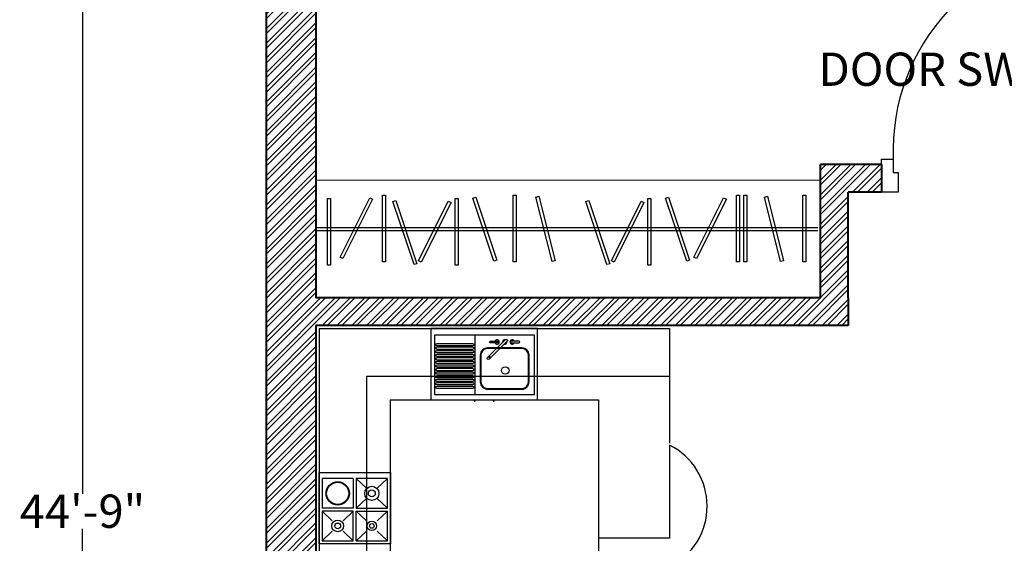
# Model space of a CAD drawing. Units: inches. Extents: x 528 to 2520, y -151 to 1354.
# Tile 2 of 41: x 542 to 720, y 1043 to 1137. Entities that reach past the tile are written whole.
import ezdxf

# ---------------------------------------------------------------- set-up
doc = ezdxf.new("R2010")
doc.units = ezdxf.units.IN
doc.header["$MEASUREMENT"] = 0
for name, color, linetype, lineweight in [('A-ANNO-DIMS', 2, 'Continuous', 18), ('A-Door', 150, 'Continuous', 25), ('A-FLOR-CASE', 11, 'Continuous', 20), ('A-WALL-PATT', 6, 'Continuous', 13), ('walls', 7, 'Continuous', 40)]:
    doc.layers.add(name, color=color, linetype=linetype, lineweight=lineweight)
for name, color, linetype in [('ESYA', 11, 'Continuous'), ('HID', 11, 'Continuous'), ('NT', 1, 'Continuous'), ('TEFRIS', 11, 'Continuous')]:
    doc.layers.add(name, color=color, linetype=linetype)
doc.styles.get("Standard").update_dxf_attribs({"font": 'arial.ttf'})
doc.dimstyles.get("Standard").update_dxf_attribs({"dimtxt": 6, "dimasz": 2, "dimexe": 0.18, "dimexo": 0.0625, "dimgap": 0.09, "dimtad": 0, "dimtih": 1, "dimtoh": 1, "dimdec": 1, "dimzin": 0, "dimdsep": 46, "dimlunit": 3, "dimtxsty": 'Standard', "dimblk": 'ARCHTICK', "dimcen": 0.09, "dimadec": 0, "dimazin": 0, "dimtfac": 1, "dimtdec": 1, "dimtofl": 0, "dimtmove": 0, "dimatfit": 3, "dimfxl": 1, "dimtolj": 1, "dimtzin": 0, "dimarcsym": 0})

# ---------------------------------------------------------------- blocks, each defined once
blk = doc.blocks.new('A$C7DB75F4D')
at = {"layer": 'A-Door'}
for points in [[(625, 740), (625, 660), (665, 660), (665, 740)], [(625, 180), (625, 660), (665, 660), (665, 180)], [(625, 100), (625, 180), (665, 180), (665, 100)], [(35, 100), (35, 60), (50, 60), (50, 50), (50, 0), (0, 0), (0, 100)], [(665, 100), (700, 100), (700, 0), (650, 0), (650, 50), (650, 60), (665, 60)]]:
    blk.add_lwpolyline(points, close=True, dxfattribs=at)
at = {"layer": 'NT'}
blk.add_arc((650, 125), 615.5, 92.3278, 182.3278, dxfattribs=at)
blk = doc.blocks.new('A$C41BE763B')
at = {"layer": 'HID'}
for p, q in [((3.395, 0.2532), (0, 0.2532)), ((3.395, 0.2332), (0, 0.2332))]:
    blk.add_line(p, q, dxfattribs=at)
for points in [[(0.4716, 0.4734), (0.4716, 0.0234), (0.4508, 0.0234), (0.4508, 0.4734)], [(1.3547, 0.4734), (1.3547, 0.0234), (1.3339, 0.0234), (1.3339, 0.4734)], [(2.8639, 0.4734), (2.8639, 0.0234), (2.8432, 0.0234), (2.8432, 0.4734)], [(2.9139, 0.4734), (2.9139, 0.0234), (2.8932, 0.0234), (2.8932, 0.4734)], [(3.3139, 0.4734), (3.3139, 0.0234), (3.2932, 0.0234), (3.2932, 0.4734)], [(0.0983, 0.45), (0.0983, 0), (0.0775, 0), (0.0775, 0.45)], [(0.3834, 0.447), (0.1822, 0.0445), (0.1636, 0.0538), (0.3648, 0.4563)], [(0.5408, 0.4372), (0.6831, 0.0103), (0.6634, 0.0037), (0.5211, 0.4306)], [(0.914, 0.4236), (0.7128, 0.0211), (0.6942, 0.0304), (0.8954, 0.4329)], [(0.9617, 0.45), (0.9617, 0), (0.941, 0), (0.941, 0.45)], [(1.0809, 0.4606), (1.2232, 0.0337), (1.2035, 0.0271), (1.0612, 0.454)], [(1.5084, 0.466), (1.6175, 0.0294), (1.5974, 0.0244), (1.4882, 0.4609)], [(1.8448, 0.4372), (1.9871, 0.0103), (1.9674, 0.0037), (1.8251, 0.4306)], [(2.218, 0.4236), (2.0167, 0.0211), (1.9981, 0.0304), (2.1994, 0.4329)], [(2.2657, 0.45), (2.2657, 0), (2.2449, 0), (2.2449, 0.45)], [(2.3849, 0.4606), (2.5272, 0.0337), (2.5075, 0.0271), (2.3652, 0.454)], [(2.7757, 0.447), (2.5745, 0.0445), (2.5559, 0.0538), (2.7572, 0.4563)], [(3.0533, 0.466), (3.1624, 0.0294), (3.1423, 0.0244), (3.0332, 0.4609)]]:
    blk.add_lwpolyline(points, close=True, dxfattribs=at)
blk = doc.blocks.new('AR365L')
blk.add_line((0, 0.0995), (0.61, 0.0995))
blk.add_lwpolyline([(0, 0), (0, 0.68), (0.61, 0.68), (0.61, 0)], close=True)
blk = doc.blocks.new('FIRIN1')
at = {"layer": 'ESYA'}
for p, q in [((0.2875, -0.05), (0.2875, -0.3006)), ((0.3983, -0.1319), (0.3125, -0.05)), ((0.575, -0.05), (0.4892, -0.1319)), ((0.3983, -0.2187), (0.3125, -0.3006)), ((0.575, -0.3006), (0.4892, -0.2187)), ((0.2875, -0.3006), (0.025, -0.3006)), ((0.025, -0.3244), (0.1108, -0.4063)), ((0.2017, -0.4063), (0.2875, -0.3244)), ((0.3983, -0.4063), (0.3125, -0.3244)), ((0.575, -0.3244), (0.4892, -0.4063)), ((0.025, -0.575), (0.1108, -0.4931)), ((0.2017, -0.4931), (0.2875, -0.575)), ((0.3983, -0.4931), (0.3125, -0.575)), ((0.575, -0.575), (0.4892, -0.4931))]:
    blk.add_line(p, q, dxfattribs=at)
blk.add_lwpolyline([(0, 0), (0.6, 0), (0.6, -0.6), (0, -0.6)], close=True, dxfattribs=at)
for points in [[(0.2875, -0.05), (0.025, -0.05), (0.025, -0.3006)], [(0.3125, -0.05), (0.3125, -0.3006), (0.575, -0.3006)], [(0.575, -0.3006), (0.575, -0.05), (0.3125, -0.05)], [(0.2875, -0.575), (0.2875, -0.3244), (0.025, -0.3244)], [(0.025, -0.3244), (0.025, -0.575)], [(0.3125, -0.575), (0.3125, -0.3244), (0.575, -0.3244)], [(0.3125, -0.575), (0.575, -0.575), (0.575, -0.3244)], [(0.025, -0.575), (0.2875, -0.575)]]:
    blk.add_lwpolyline(points, dxfattribs=at)
for centre, radius in [((0.1562, -0.1753), 0.0986), ((0.1562, -0.1753), 0.0936), ((0.4438, -0.1753), 0.0597), ((0.4438, -0.1753), 0.0294), ((0.1562, -0.4497), 0.0492), ((0.4438, -0.4497), 0.0398), ((0.1562, -0.4497), 0.0242), ((0.4438, -0.4497), 0.0196)]:
    blk.add_circle(centre, radius, dxfattribs=at)
blk = doc.blocks.new('ncvn')
for p, q in [((77868.38, -4466.7), (77868.38, -4520.7)), ((77949.38, -4466.7), (77868.38, -4466.7)), ((77949.38, -4520.7), (77949.38, -4466.7))]:
    blk.add_line(p, q)
at = {"layer": 'TEFRIS'}
for p, q in [((77783.66, -4466.69), (77783.66, -4763.38)), ((77783.66, -4466.69), (78049.52, -4466.69)), ((77901.95, -4516.62), (77901.95, -4471.62)), ((78049.52, -4466.69), (78049.52, -4553.55)), ((77819.66, -4502.83), (77819.66, -4759.23)), ((77819.66, -4502.83), (78049.52, -4502.83)), ((77837.66, -4520.83), (77837.66, -4704.71)), ((77837.66, -4520.83), (77995.52, -4520.83)), ((77868.38, -4520.7), (77949.38, -4520.7)), ((77995.52, -4520.83), (77995.52, -4642.99)), ((78049.52, -4554.99), (78049.52, -4625.66)), ((78049.52, -4625.66), (77995.83, -4625.66)), ((77783.66, -4704.71), (77837.66, -4704.71))]:
    blk.add_line(p, q, dxfattribs=at)
for points in [[(77868.38, -4466.7), (77868.38, -4520.7), (77949.38, -4520.7), (77949.38, -4466.7)], [(77871.35, -4471.62), (77871.35, -4516.62), (77946.95, -4516.62), (77946.95, -4471.62)]]:
    blk.add_lwpolyline(points, close=True, dxfattribs=at)
for points in [[(77873.15, -4477.92), (77900.15, -4477.92, -1), (77900.15, -4479.72), (77873.15, -4479.72, -1), (77873.15, -4477.92)], [(77873.15, -4480.62), (77900.15, -4480.62, -1), (77900.15, -4482.42), (77873.15, -4482.42, -1), (77873.15, -4480.62)], [(77873.15, -4483.32), (77900.15, -4483.32, -1), (77900.15, -4485.12), (77873.15, -4485.12, -1), (77873.15, -4483.32)], [(77873.15, -4486.02), (77900.15, -4486.02, -1), (77900.15, -4487.82), (77873.15, -4487.82, -1), (77873.15, -4486.02)], [(77873.15, -4488.72), (77900.15, -4488.72, -1), (77900.15, -4490.52), (77873.15, -4490.52, -1), (77873.15, -4488.72)], [(77873.15, -4491.42), (77900.15, -4491.42, -1), (77900.15, -4493.22), (77873.15, -4493.22, -1), (77873.15, -4491.42)], [(77873.15, -4494.12), (77900.15, -4494.12, -1), (77900.15, -4495.92), (77873.15, -4495.92, -1), (77873.15, -4494.12)], [(77873.15, -4496.82), (77900.15, -4496.82, -1), (77900.15, -4498.62), (77873.15, -4498.62, -1), (77873.15, -4496.82)], [(77873.15, -4499.52), (77900.15, -4499.52, -1), (77900.15, -4501.32), (77873.15, -4501.32, -1), (77873.15, -4499.52)], [(77873.15, -4502.22), (77900.15, -4502.22, -1), (77900.15, -4504.02), (77873.15, -4504.02, -1), (77873.15, -4502.22)], [(77873.15, -4504.92), (77900.15, -4504.92, -1), (77900.15, -4506.72), (77873.15, -4506.72, -1), (77873.15, -4504.92)], [(77873.15, -4507.62), (77900.15, -4507.62, -1), (77900.15, -4509.42), (77873.15, -4509.42, -1), (77873.15, -4507.62)], [(77873.15, -4510.32), (77900.15, -4510.32, -1), (77900.15, -4512.12), (77873.15, -4512.12, -1), (77873.15, -4510.32)]]:
    blk.add_lwpolyline(points, format="xyb", dxfattribs=at)
for points in [[(77911.5, -4488.58), (77925.04, -4475.05, -1), (77926.25, -4476.26), (77912.72, -4489.8, -1)], [(77913.54, -4476.29), (77919.71, -4476.29, -0.563183), (77919.71, -4477.44), (77913.54, -4477.44, -1)], [(77935.33, -4476.29), (77929.17, -4476.29, 0.563183), (77929.17, -4477.44), (77935.33, -4477.44, 1)], [(77905.95, -4486.73), (77905.95, -4507.22, 0.414214), (77911.35, -4512.62), (77937.55, -4512.62, 0.414214), (77942.95, -4507.22), (77942.95, -4486.73, 0.414214), (77937.55, -4481.33), (77911.35, -4481.33, 0.414214)], [(77906.49, -4486.73), (77906.49, -4507.22, 0.414214), (77911.35, -4512.08), (77937.55, -4512.08, 0.414214), (77942.41, -4507.22), (77942.41, -4486.73, 0.414214), (77937.55, -4481.87), (77911.35, -4481.87, 0.414214)]]:
    blk.add_lwpolyline(points, format="xyb", close=True, dxfattribs=at)
for points in [[(77901.23, -4520.7), (77901.23, -4521.6), (77902.13, -4521.6), (77902.13, -4520.7)], [(77915.63, -4520.7), (77915.63, -4521.6), (77916.53, -4521.6), (77916.53, -4520.7)]]:
    blk.add_lwpolyline(points, dxfattribs=at)
for centre, radius in [((77913.01, -4488.3), 0.571), ((77924.89, -4498.48), 2.86)]:
    blk.add_circle(centre, radius, dxfattribs=at)
for centre, radius, start, end in [((77918.69, -4476.87), 1.71, 199.47122, 160.52878), ((77924.44, -4476.87), 1.71, 75, 195), ((77924.44, -4476.87), 1.71, 255, 15), ((77930.19, -4476.87), 1.71, 19.47122, 340.52878), ((78026.22, -4601.26), 51.8, 233.6588, 63.26709)]:
    blk.add_arc(centre, radius, start, end, dxfattribs=at)
at = {"layer": 'TEFRIS', "xscale": 90, "yscale": 90, "zscale": 90}
blk.add_blockref('FIRIN1', (77783.76, -4575.88), dxfattribs=at)
at = {"layer": 'TEFRIS', "xscale": 90, "yscale": 90, "zscale": 90, "rotation": 90}
blk.add_blockref('AR365L', (77848.22, -4760.91), dxfattribs=at)
blk = doc.blocks.new('_ArchTick')
at = {"color": 0, "linetype": 'ByBlock', "const_width": 0.15}
blk.add_lwpolyline([(-0.5, -0.5), (0.5, 0.5)], dxfattribs=at)
blk = doc.blocks.new('*D40')
at = {"layer": 'A-ANNO-DIMS', "color": 0, "lineweight": -2, "transparency": 16777216}
for p, q in [((744.63, 1150.5), (737.86, 1150.5)), ((738.04, 1150.5), (738.04, 1131.5)), ((738.04, 1106.1), (738.04, 1125.11)), ((744.63, 1106.1), (737.86, 1106.1))]:
    blk.add_line(p, q, dxfattribs=at)
at = {"layer": 'Defpoints', "color": 0, "transparency": 16777216}
for p in [(738.04, 1150.5), (744.7, 1150.5), (744.7, 1106.1)]:
    blk.add_point(p, dxfattribs=at)
at = {"layer": 'A-ANNO-DIMS', "color": 0, "lineweight": -2, "transparency": 16777216, "xscale": 2, "yscale": 2, "zscale": 2}
for p, rotation in [((738.04, 1150.5), 90), ((738.04, 1106.1), 270)]:
    blk.add_blockref('_ArchTick', p, dxfattribs=dict(at, rotation=rotation))
at = {"layer": 'A-ANNO-DIMS', "color": 0, "transparency": 16777216, "insert": (738.04, 1128.3), "char_height": 6, "attachment_point": 5}
blk.add_mtext('\\A1;DOOR SWING 3\'-8 1/2" TYP.', dxfattribs=at)
blk = doc.blocks.new('*D92')
at = {"layer": 'A-ANNO-DIMS', "color": 0, "lineweight": -2, "transparency": 16777216}
for p, q in [((586.63, 1317.1), (553.42, 1317.1)), ((553.6, 1317.1), (553.6, 1051.76)), ((553.6, 780.1), (553.6, 1045.45)), ((586.63, 780.1), (553.42, 780.1))]:
    blk.add_line(p, q, dxfattribs=at)
at = {"layer": 'Defpoints', "color": 0, "transparency": 16777216}
for p in [(553.6, 1317.1), (586.7, 1317.1), (586.7, 780.1)]:
    blk.add_point(p, dxfattribs=at)
at = {"layer": 'A-ANNO-DIMS', "color": 0, "lineweight": -2, "transparency": 16777216, "xscale": 2, "yscale": 2, "zscale": 2}
for p, rotation in [((553.6, 1317.1), 90), ((553.6, 780.1), 270)]:
    blk.add_blockref('_ArchTick', p, dxfattribs=dict(at, rotation=rotation))
at = {"layer": 'A-ANNO-DIMS', "color": 0, "transparency": 16777216, "insert": (553.6, 1048.6), "char_height": 6, "attachment_point": 5}
blk.add_mtext('\\A1;44\'-9"', dxfattribs=at)

msp = doc.modelspace()

# ---------------------------------------------------------------- hatches: boundary and pattern name
at = {"layer": 'A-WALL-PATT'}
h = msp.add_hatch(dxfattribs=at)
h.set_pattern_fill('ANSI32', color=256, scale=5)
h.paths.add_polyline_path([(595.7, 1163.86), (586.7, 1163.86), (586.7, 969.1), (598.24, 969.1), (603.24, 969.1), (603.24, 974.1), (595.7, 974.1), (595.7, 1082.1), (691.7, 1082.1), (691.7, 1087.1), (691.7, 1106.1), (697.7, 1106.1), (697.7, 1111.1), (686.7, 1111.1), (686.7, 1087.1), (595.7, 1087.1)])
h.paths.add_polyline_path([(688.7, 974.1), (651.24, 974.1), (651.24, 969.1), (688.7, 969.1)])
h.paths.add_polyline_path([(885.7, 1171.37), (876.7, 1171.37), (876.7, 1111.1), (786.7, 1111.1), (786.7, 1106.1), (876.7, 1106.1), (876.7, 974.1), (786.7, 974.1), (786.7, 969.1), (876.7, 969.1), (876.7, 825.1), (834.7, 825.1), (834.7, 816.1), (885.7, 816.1)])
h.paths.add_polyline_path([(885.7, 1317.1), (876.65, 1317.1), (876.65, 1308.1), (876.7, 1308.1), (876.7, 1248.1), (822.7, 1248.1), (822.7, 1243.1), (876.7, 1243.1), (876.7, 1219.37), (885.7, 1219.37)])
h.paths.add_polyline_path([(852.65, 1317.1), (787.7, 1317.1), (787.7, 1248.1), (784.26, 1248.1), (784.26, 1243.1), (792.7, 1243.1), (792.7, 1249.1), (792.7, 1308.1), (852.65, 1308.1)])
h.paths.add_polyline_path([(684.7, 1317.1), (619.7, 1317.1), (619.7, 1308.1), (679.7, 1308.1), (679.7, 1248.1), (679.7, 1243.1), (684.7, 1243.1), (684.7, 1248.25)])
h.paths.add_polyline_path([(595.7, 1308.1), (595.7, 1317.1), (586.7, 1317.1), (586.7, 1211.86), (595.7, 1211.86), (595.7, 1243.1), (649.7, 1243.1), (649.7, 1248.1), (595.7, 1248.1)])
h.paths.add_polyline_path([(744.7, 969.1), (744.7, 974.1), (724.7, 974.1), (724.7, 969.1), (739.7, 969.1), (739.7, 874.29), (744.7, 874.29)])
h.paths.add_polyline_path([(739.7, 969.1), (727.7, 969.1), (727.7, 965.12), (730.74, 965.12), (730.74, 961.68), (734.43, 961.68), (734.43, 957.24), (739.7, 957.24)], flags=17)
h.paths.add_polyline_path([(786.7, 825.1), (744.7, 825.1), (744.7, 832.29), (739.7, 832.29), (739.7, 816.1), (786.7, 816.1)])

# ---------------------------------------------------------------- linework, layer by layer
at = {"layer": 'A-FLOR-CASE'}
msp.add_line((595.7, 1108.27), (686.7, 1108.27), dxfattribs=at)
at = {"layer": 'walls'}
for p, q in [((586.7, 1317.1), (586.7, 789.1)), ((595.7, 1243.1), (595.7, 1087.1)), ((686.7, 1087.1), (686.7, 1111.1)), ((697.7, 1111.1), (686.7, 1111.1)), ((697.7, 1111.1), (697.7, 1106.1)), ((691.7, 1087.1), (691.7, 1106.1)), ((697.7, 1106.1), (691.7, 1106.1)), ((686.7, 1087.1), (595.7, 1087.1)), ((691.7, 1087.1), (691.7, 1082.1)), ((691.7, 1082.1), (595.7, 1082.1)), ((595.7, 1082.1), (595.7, 974.1))]:
    msp.add_line(p, q, dxfattribs=at)

# ---------------------------------------------------------------- block references
at = {"layer": 'A-Door', "xscale": 0.0600000000000059, "yscale": 0.0600000000000059, "zscale": 0.0600000000000059}
msp.add_blockref('A$C7DB75F4D', (697.7, 1106.1), dxfattribs=at)
at = {"layer": 'A-FLOR-CASE'}
for name, p, xscale, yscale, zscale in [('A$C41BE763B', (595.7, 1092.96), 26.66231123505322, 26.66231123505322, 26.66231123505322), ('ncvn', (-17896.58, 2143.47), 0.2377471155606993, 0.2377471155606993, 0.2377471155606993)]:
    msp.add_blockref(name, p, dxfattribs=dict(at, xscale=xscale, yscale=yscale, zscale=zscale))

# ---------------------------------------------------------------- dimensions: what is measured, and where the dimension line sits
at = {"layer": 'A-ANNO-DIMS'}
dim = msp.add_linear_dim(base=(553.6, 1317.1), p1=(586.7, 780.1), p2=(586.7, 1317.1), angle=90, dimstyle='Standard', override={"dimdec": 1, "dimlfac": 1, "dimrnd": 0, "dimzin": 1, "dimdsep": 46, "dimlunit": 4, "dimfrac": 2}, dxfattribs=at)
dim.commit()
dim.dimension.update_dxf_attribs({"geometry": '*D92', "text_midpoint": (553.6, 1048.6)})
dim = msp.add_linear_dim(base=(738.04, 1150.5), p1=(744.7, 1106.1), p2=(744.7, 1150.5), angle=90, text='DOOR SWING <> TYP.', dimstyle='Standard', override={"dimdec": 1, "dimlfac": 1, "dimrnd": 0, "dimzin": 1, "dimdsep": 46, "dimlunit": 4, "dimfrac": 2}, dxfattribs=at)
dim.commit()
dim.dimension.update_dxf_attribs({"geometry": '*D40', "text_midpoint": (738.04, 1128.3)})

doc.saveas('drawing.dxf')
